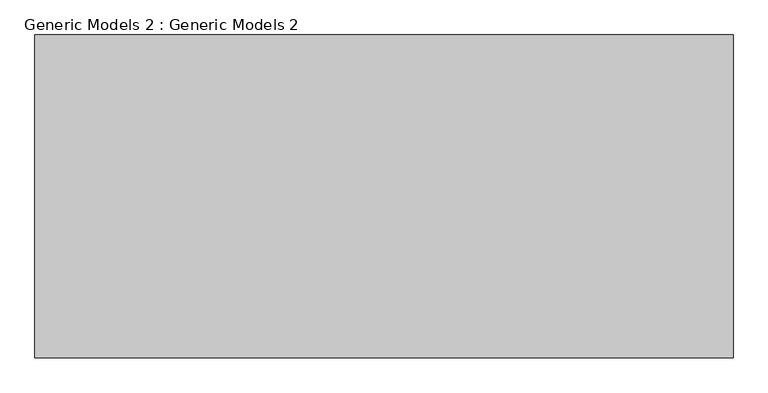
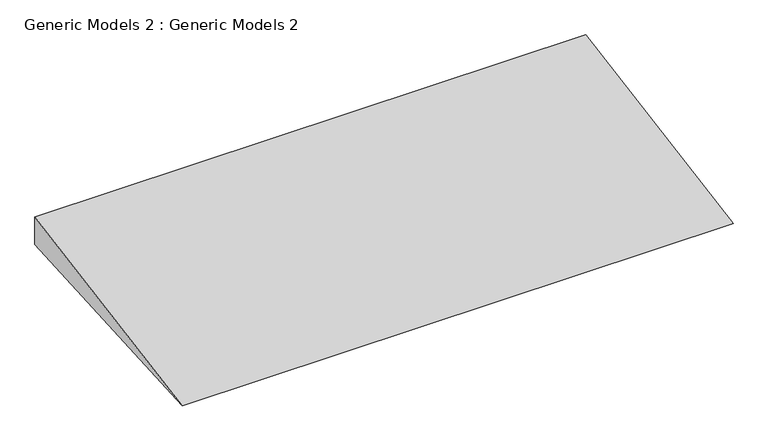
"""IFC4 building model written with IfcOpenShell, lengths in millimetres: proxy geometry, Generic Models 2 : Generic Models 2."""

from ifc_helpers import new_model, si_unit, frame, origin, place, context, project, spatial, polyline, outline, extrude, source, transform, mapped, element, save


def generic_models_2_generic_models_2_e98e430d(model_context):
    return source(origin(), model_context, "Body", "SweptSolid", [
        extrude(outline(polyline([(-15017.1711839, -238.1758405), (-13666.4088699, 0.0), (-13666.4088699, -152.4336369), (-15017.1711839, -238.1758405)])), frame((-3098.7352229, 0.0, 0.0), z_axis=(1.0, 0.0, 0.0), x_axis=(0.0, 1.0, 0.0)), (0.0, 0.0, 1.0), 2920.0519506),
    ])


if __name__ == "__main__":
    model = new_model("IFC4")
    model_context = context("Model", 3, world=origin())
    ifc_project = project(units=[si_unit("LENGTHUNIT", "METRE", prefix="MILLI")], contexts=[model_context])
    site = spatial("IfcSite", under=ifc_project)
    building = spatial("IfcBuilding", under=site)
    placement = place(None, origin())
    generic_models_2_generic_models_2_shape = generic_models_2_generic_models_2_e98e430d(model_context)
    element("IfcBuildingElementProxy", 1, Name="Generic Models 2 : Generic Models 2", ObjectType="Generic Models 2 : Generic Models 2", at=placement, inside=building, context=model_context, shape_type="MappedRepresentation", body=[
        mapped(generic_models_2_generic_models_2_shape, transform((0.0, 0.0, 0.0), x_axis=(1.0, 0.0, 0.0), y_axis=(0.0, 1.0, 0.0), z_axis=(0.0, 0.0, 1.0))),
    ])
    save(model, "model.ifc")
